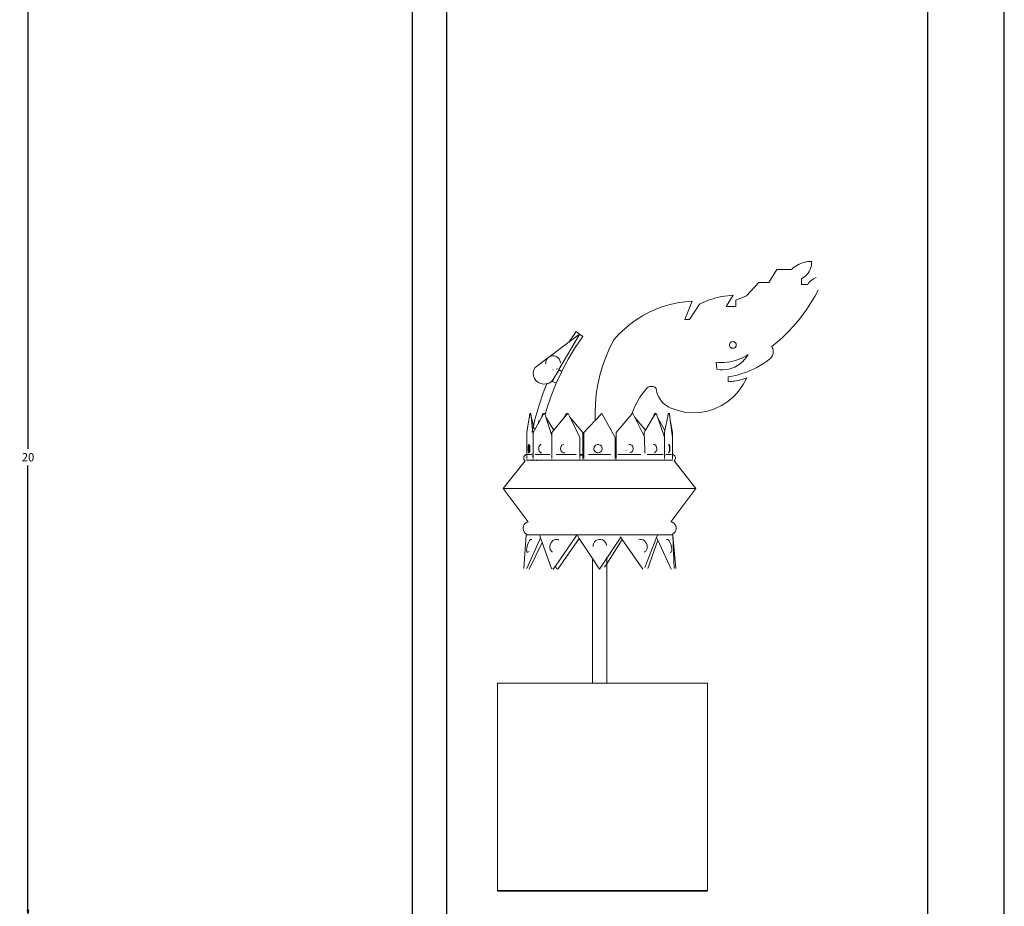
# Model space of a CAD drawing. Units: millimetres. Extents: x 446512 to 447461, y 70395 to 70610.
# Tile 4 of 39: x 446678.04 to 446699.43, y 70453.63 to 70472.88. Entities that reach past the tile are written whole.
import ezdxf

# ---------------------------------------------------------------- set-up
doc = ezdxf.new("R2010")
doc.units = ezdxf.units.MM
for name, color, linetype, lineweight in [('A-ANNO-DIMS', 2, 'Continuous', 18), ('A-FURN', 7, 'Continuous', 35), ('A-FURN-DECO', 8, 'Continuous', 13)]:
    doc.layers.add(name, color=color, linetype=linetype, lineweight=lineweight)
doc.styles.get("Standard").update_dxf_attribs({"font": 'arial.ttf'})
doc.dimstyles.get("Standard").update_dxf_attribs({"dimtxt": 0.18, "dimasz": 0.18, "dimexe": 0.18, "dimexo": 0.0625, "dimgap": 0.09, "dimtad": 0, "dimtih": 1, "dimtoh": 1, "dimdec": 4, "dimzin": 0, "dimdsep": 46, "dimtxsty": 'Standard', "dimcen": 0.09, "dimadec": 0, "dimazin": 0, "dimtfac": 1, "dimtdec": 4, "dimtofl": 0, "dimtmove": 0, "dimatfit": 3, "dimfxl": 1, "dimtolj": 1, "dimtzin": 0, "dimarcsym": 0})

# ---------------------------------------------------------------- blocks, each defined once
blk = doc.blocks.new('*D20')
at = {"layer": 'A-ANNO-DIMS', "color": 0, "lineweight": -2, "transparency": 16777216}
for p, q in [((446686.51, 70473.382), (446678.043, 70473.382)), ((446678.223, 70473.202), (446678.223, 70463.563)), ((446678.223, 70453.562), (446678.223, 70463.2)), ((446686.51, 70453.382), (446678.043, 70453.382))]:
    blk.add_line(p, q, dxfattribs=at)
at = {"layer": 'A-ANNO-DIMS', "color": 0, "transparency": 16777216}
for points in [[(446678.193, 70473.202), (446678.253, 70473.202), (446678.223, 70473.382)], [(446678.193, 70453.562), (446678.253, 70453.562), (446678.223, 70453.382)]]:
    blk.add_solid(points, dxfattribs=at)
at = {"layer": 'Defpoints', "color": 0, "transparency": 16777216}
for p in [(446678.223, 70473.382), (446686.573, 70473.382), (446686.573, 70453.382)]:
    blk.add_point(p, dxfattribs=at)
at = {"layer": 'A-ANNO-DIMS', "color": 0, "transparency": 16777216, "insert": (446678.223, 70463.382), "char_height": 0.18, "attachment_point": 5}
blk.add_mtext('\\A1;20', dxfattribs=at)
blk = doc.blocks.new('*D37')
at = {"layer": 'A-ANNO-DIMS', "color": 0, "lineweight": -2, "transparency": 16777216}
for p, q in [((446686.572846, 70433.44405), (446686.572846, 70578.17492)), ((446687.323552, 70428.838404), (446687.323552, 70578.17492)), ((446686.392846, 70577.99492), (446686.212846, 70577.99492)), ((446687.503552, 70577.99492), (446687.683552, 70577.99492))]:
    blk.add_line(p, q, dxfattribs=at)
at = {"layer": 'A-ANNO-DIMS', "color": 0, "transparency": 16777216}
for points in [[(446686.392846, 70578.02492), (446686.392846, 70577.96492), (446686.572846, 70577.99492)], [(446687.503552, 70578.02492), (446687.503552, 70577.96492), (446687.323552, 70577.99492)]]:
    blk.add_solid(points, dxfattribs=at)
at = {"layer": 'Defpoints', "color": 0, "transparency": 16777216}
for p in [(446687.323552, 70577.99492), (446686.572846, 70433.38155), (446687.323552, 70428.775904)]:
    blk.add_point(p, dxfattribs=at)
at = {"layer": 'A-ANNO-DIMS', "color": 0, "transparency": 16777216, "insert": (446686.948199, 70577.99492), "char_height": 0.18, "attachment_point": 5}
blk.add_mtext('\\A1;0.75', dxfattribs=at)
blk = doc.blocks.new('*D38')
at = {"layer": 'A-ANNO-DIMS', "color": 0, "lineweight": -2, "transparency": 16777216}
for p, q in [((446687.323552, 70428.838404), (446687.323552, 70578.17492)), ((446697.765686, 70428.838404), (446697.765686, 70578.17492)), ((446687.503552, 70577.99492), (446692.090383, 70577.99492)), ((446697.585686, 70577.99492), (446692.998855, 70577.99492))]:
    blk.add_line(p, q, dxfattribs=at)
at = {"layer": 'A-ANNO-DIMS', "color": 0, "transparency": 16777216}
for points in [[(446687.503552, 70578.02492), (446687.503552, 70577.96492), (446687.323552, 70577.99492)], [(446697.585686, 70578.02492), (446697.585686, 70577.96492), (446697.765686, 70577.99492)]]:
    blk.add_solid(points, dxfattribs=at)
at = {"layer": 'Defpoints', "color": 0, "transparency": 16777216}
for p in [(446697.765686, 70577.99492), (446687.323552, 70428.775904), (446697.765686, 70428.775904)]:
    blk.add_point(p, dxfattribs=at)
at = {"layer": 'A-ANNO-DIMS', "color": 0, "transparency": 16777216, "insert": (446692.544619, 70577.99492), "char_height": 0.18, "attachment_point": 5}
blk.add_mtext('\\A1;10.442', dxfattribs=at)
blk = doc.blocks.new('*D39')
at = {"layer": 'A-ANNO-DIMS', "color": 0, "lineweight": -2, "transparency": 16777216}
for p, q in [((446697.766, 70428.838), (446697.766, 70578.175)), ((446699.429, 70433.444), (446699.429, 70578.175)), ((446697.946, 70577.995), (446698.212, 70577.995)), ((446699.249, 70577.995), (446698.982, 70577.995))]:
    blk.add_line(p, q, dxfattribs=at)
at = {"layer": 'A-ANNO-DIMS', "color": 0, "transparency": 16777216}
for points in [[(446697.946, 70578.025), (446697.946, 70577.965), (446697.766, 70577.995)], [(446699.249, 70578.025), (446699.249, 70577.965), (446699.429, 70577.995)]]:
    blk.add_solid(points, dxfattribs=at)
at = {"layer": 'Defpoints', "color": 0, "transparency": 16777216}
for p in [(446699.429, 70577.995), (446699.429, 70433.382), (446697.766, 70428.776)]:
    blk.add_point(p, dxfattribs=at)
at = {"layer": 'A-ANNO-DIMS', "color": 0, "transparency": 16777216, "insert": (446698.597, 70577.995), "char_height": 0.18, "attachment_point": 5}
blk.add_mtext('\\A1;1.663', dxfattribs=at)

msp = doc.modelspace()

# ---------------------------------------------------------------- linework, layer by layer
at = {"layer": 'A-FURN'}
msp.add_line((446688.42, 70453.9655), (446692.9826, 70453.9655), dxfattribs=at)
at = {"layer": 'A-FURN-DECO'}
for p, q in [((446694.3144, 70467.1785), (446694.4873, 70467.4578)), ((446694.4873, 70467.4578), (446694.8067, 70467.4578)), ((446694.8067, 70467.4578), (446694.8365, 70467.4847)), ((446694.8365, 70467.4847), (446694.8679, 70467.5096)), ((446694.8679, 70467.5096), (446694.9009, 70467.5324)), ((446694.9009, 70467.5324), (446694.9353, 70467.5531)), ((446694.9353, 70467.5531), (446694.9709, 70467.5716)), ((446694.9709, 70467.5716), (446695.0077, 70467.5878)), ((446695.0077, 70467.5878), (446695.0454, 70467.6015)), ((446695.0454, 70467.6015), (446695.0839, 70467.6129)), ((446695.0839, 70467.6129), (446695.123, 70467.6217)), ((446695.123, 70467.6217), (446695.1627, 70467.6281)), ((446695.1627, 70467.6281), (446695.2026, 70467.6319)), ((446695.2053, 70467.4459), (446695.1875, 70467.4117)), ((446695.2026, 70467.6319), (446695.2427, 70467.6331)), ((446695.2199, 70467.4816), (446695.2053, 70467.4459)), ((446695.2309, 70467.5185), (446695.2199, 70467.4816)), ((446695.2385, 70467.5562), (446695.2309, 70467.5185)), ((446695.2424, 70467.5946), (446695.2385, 70467.5562)), ((446695.2427, 70467.6331), (446695.2424, 70467.5946)), ((446695.0554, 70467.274), (446695.022, 70467.2548)), ((446695.022, 70467.2548), (446695.022, 70467.1316)), ((446695.0868, 70467.2963), (446695.0554, 70467.274)), ((446695.116, 70467.3214), (446695.0868, 70467.2963)), ((446695.1426, 70467.3492), (446695.116, 70467.3214)), ((446695.1666, 70467.3794), (446695.1426, 70467.3492)), ((446695.1875, 70467.4117), (446695.1666, 70467.3794)), ((446695.2254, 70467.2123), (446695.2525, 70467.2346)), ((446695.2525, 70467.2346), (446695.2816, 70467.2541)), ((446695.2816, 70467.2541), (446695.3124, 70467.2707)), ((446695.3124, 70467.2707), (446695.3446, 70467.2842)), ((446693.8287, 70466.8825), (446694.0999, 70467.1785)), ((446694.0999, 70467.1785), (446694.3144, 70467.1785)), ((446695.022, 70467.1316), (446695.1589, 70467.1316)), ((446695.1589, 70467.1316), (446695.1784, 70467.1606)), ((446695.1784, 70467.1606), (446695.2007, 70467.1876)), ((446695.2007, 70467.1876), (446695.2254, 70467.2123)), ((446692.9818, 70466.7815), (446693.042, 70466.8034)), ((446693.042, 70466.8034), (446693.1028, 70466.8231)), ((446693.1028, 70466.8231), (446693.1644, 70466.8406)), ((446693.1644, 70466.8406), (446693.2265, 70466.8559)), ((446693.2265, 70466.8559), (446693.2891, 70466.869)), ((446693.2891, 70466.869), (446693.3522, 70466.8798)), ((446693.3522, 70466.8798), (446693.4156, 70466.8884)), ((446693.5431, 70466.8987), (446693.3856, 70466.6528)), ((446693.4156, 70466.8884), (446693.4793, 70466.8947)), ((446693.4793, 70466.8947), (446693.5431, 70466.8987)), ((446693.5955, 70466.7897), (446693.8287, 70466.8825)), ((446695.3111, 70466.8693), (446695.2297, 70466.7314)), ((446695.3861, 70467.0106), (446695.3111, 70466.8693)), ((446691.7134, 70466.5282), (446691.8616, 70466.5952)), ((446691.8616, 70466.5952), (446692.014, 70466.6519)), ((446692.014, 70466.6519), (446692.1699, 70466.6981)), ((446692.1699, 70466.6981), (446692.3286, 70466.7337)), ((446692.3286, 70466.7337), (446692.4893, 70466.7584)), ((446692.4893, 70466.7584), (446692.6513, 70466.7721)), ((446692.6513, 70466.7721), (446692.4922, 70466.3689)), ((446692.5926, 70466.3689), (446692.8067, 70466.7032)), ((446692.8067, 70466.7032), (446692.8641, 70466.7314)), ((446692.8641, 70466.7314), (446692.9225, 70466.7575)), ((446692.9225, 70466.7575), (446692.9818, 70466.7815)), ((446693.3856, 70466.6528), (446693.5955, 70466.6528)), ((446693.5955, 70466.6528), (446693.5955, 70466.7897)), ((446695.1424, 70466.5973), (446695.0491, 70466.4672)), ((446695.2297, 70466.7314), (446695.1424, 70466.5973)), ((446691.4323, 70466.365), (446691.5701, 70466.4514)), ((446691.5701, 70466.4514), (446691.7134, 70466.5282)), ((446695.0491, 70466.4672), (446694.9501, 70466.3414)), ((446691.0586, 70466.0527), (446691.176, 70466.1652)), ((446691.176, 70466.1652), (446691.3008, 70466.2695)), ((446691.3008, 70466.2695), (446691.4323, 70466.365)), ((446692.4922, 70466.3689), (446692.5926, 70466.3689)), ((446694.8456, 70466.2202), (446694.7359, 70466.1037)), ((446694.9501, 70466.3414), (446694.8456, 70466.2202)), ((446690.202, 70466.0449), (446689.7562, 70465.2847)), ((446690.1268, 70466.1082), (446689.9751, 70465.8868)), ((446690.202, 70466.0567), (446689.9751, 70465.8868)), ((446690.1103, 70465.7614), (446690.2773, 70466.0051)), ((446690.202, 70466.0567), (446690.1268, 70466.1082)), ((446690.202, 70466.0449), (446690.202, 70466.0567)), ((446690.2773, 70466.0051), (446690.202, 70466.0567)), ((446690.9491, 70465.9325), (446691.0586, 70466.0527)), ((446694.621, 70465.9922), (446694.5013, 70465.886)), ((446694.7359, 70466.1037), (446694.621, 70465.9922)), ((446689.9751, 70465.8868), (446689.5362, 70465.5564)), ((446689.9581, 70465.511), (446690.1103, 70465.7614)), ((446690.8555, 70465.7475), (446690.7735, 70465.557)), ((446690.9491, 70465.9325), (446690.8555, 70465.7475)), ((446693.4621, 70465.8096), (446693.4622, 70465.8286)), ((446693.467, 70465.7911), (446693.4621, 70465.8096)), ((446693.4622, 70465.8286), (446693.4673, 70465.847)), ((446693.4764, 70465.7746), (446693.467, 70465.7911)), ((446693.4673, 70465.847), (446693.4769, 70465.8635)), ((446693.4898, 70465.761), (446693.4764, 70465.7746)), ((446693.4769, 70465.8635), (446693.4904, 70465.8769)), ((446693.5063, 70465.7514), (446693.4898, 70465.761)), ((446693.4904, 70465.8769), (446693.507, 70465.8863)), ((446693.5247, 70465.7464), (446693.5063, 70465.7514)), ((446693.507, 70465.8863), (446693.5254, 70465.8911)), ((446693.5437, 70465.7463), (446693.5247, 70465.7464)), ((446693.5254, 70465.8911), (446693.5445, 70465.891)), ((446693.5622, 70465.7511), (446693.5437, 70465.7463)), ((446693.5445, 70465.891), (446693.5628, 70465.886)), ((446693.5787, 70465.7606), (446693.5622, 70465.7511)), ((446693.5628, 70465.886), (446693.5793, 70465.8764)), ((446693.5922, 70465.774), (446693.5787, 70465.7606)), ((446693.5793, 70465.8764), (446693.5927, 70465.8629)), ((446693.6019, 70465.7904), (446693.5922, 70465.774)), ((446693.5927, 70465.8629), (446693.6022, 70465.8463)), ((446693.6069, 70465.8088), (446693.6019, 70465.7904)), ((446693.6022, 70465.8463), (446693.607, 70465.8279)), ((446693.607, 70465.8279), (446693.6069, 70465.8088)), ((446694.5013, 70465.886), (446694.3769, 70465.7852)), ((446694.3769, 70465.7852), (446694.3896, 70465.7631)), ((446694.3896, 70465.7631), (446694.3995, 70465.7396)), ((446694.3995, 70465.7396), (446694.4063, 70465.715)), ((446689.5362, 70465.5564), (446689.2354, 70465.3333)), ((446689.4825, 70465.4957), (446689.5052, 70465.5294)), ((446689.5052, 70465.5294), (446689.5362, 70465.5564)), ((446689.5362, 70465.5564), (446689.5733, 70465.5747)), ((446689.5733, 70465.5747), (446689.6141, 70465.583)), ((446689.6141, 70465.583), (446689.6557, 70465.5809)), ((446689.6557, 70465.5809), (446689.6954, 70465.5684)), ((446689.6954, 70465.5684), (446689.7303, 70465.5465)), ((446689.7303, 70465.5465), (446689.7582, 70465.5166)), ((446690.7735, 70465.557), (446690.7035, 70465.3618)), ((446693.7029, 70465.524), (446693.6465, 70465.5011)), ((446693.758, 70465.5502), (446693.7029, 70465.524)), ((446693.8114, 70465.5795), (446693.758, 70465.5502)), ((446693.8278, 70465.5548), (446693.7869, 70465.5017)), ((446693.8629, 70465.612), (446693.8114, 70465.5795)), ((446693.8629, 70465.612), (446693.8278, 70465.5548)), ((446694.3503, 70465.5275), (446694.3311, 70465.5107)), ((446694.3673, 70465.5465), (446694.3503, 70465.5275)), ((446694.3817, 70465.5675), (446694.3673, 70465.5465)), ((446694.3934, 70465.5902), (446694.3817, 70465.5675)), ((446694.4023, 70465.6141), (446694.3934, 70465.5902)), ((446694.408, 70465.6389), (446694.4023, 70465.6141)), ((446694.4063, 70465.715), (446694.4101, 70465.6898)), ((446694.4106, 70465.6643), (446694.408, 70465.6389)), ((446694.4101, 70465.6898), (446694.4106, 70465.6643)), ((446689.2354, 70465.3333), (446689.2086, 70465.2796)), ((446689.4674, 70465.4172), (446689.4696, 70465.4574)), ((446689.4677, 70465.4158), (446689.4674, 70465.4172)), ((446689.4674, 70465.4101), (446689.4677, 70465.4158)), ((446689.4696, 70465.4574), (446689.4825, 70465.4957)), ((446689.7582, 70465.5166), (446689.7771, 70465.4807)), ((446689.7771, 70465.4807), (446689.7858, 70465.4413)), ((446689.7855, 70465.4356), (446689.7858, 70465.4413)), ((446689.7855, 70465.4356), (446689.7858, 70465.4342)), ((446689.9581, 70465.511), (446689.8195, 70465.2529)), ((446690.7035, 70465.3618), (446690.6456, 70465.1627)), ((446693.2276, 70465.4378), (446693.1668, 70465.443)), ((446693.1668, 70465.443), (446693.1818, 70465.2914)), ((446693.2885, 70465.4362), (446693.2276, 70465.4378)), ((446693.3494, 70465.4382), (446693.2885, 70465.4362)), ((446693.4101, 70465.4437), (446693.3494, 70465.4382)), ((446693.4703, 70465.4528), (446693.4101, 70465.4437)), ((446693.5127, 70465.3149), (446693.4483, 70465.2963)), ((446693.53, 70465.4654), (446693.4703, 70465.4528)), ((446693.5748, 70465.3403), (446693.5127, 70465.3149)), ((446693.5887, 70465.4816), (446693.53, 70465.4654)), ((446693.6339, 70465.372), (446693.5748, 70465.3403)), ((446693.6465, 70465.5011), (446693.5887, 70465.4816)), ((446693.6894, 70465.4098), (446693.6339, 70465.372)), ((446693.7406, 70465.4532), (446693.6894, 70465.4098)), ((446693.7869, 70465.5017), (446693.7406, 70465.4532)), ((446694.0548, 70465.3329), (446693.9814, 70465.2959)), ((446694.1266, 70465.373), (446694.0548, 70465.3329)), ((446694.1967, 70465.416), (446694.1266, 70465.373)), ((446694.2649, 70465.4619), (446694.1967, 70465.416)), ((446694.3311, 70465.5107), (446694.2649, 70465.4619)), ((446689.2086, 70465.2796), (446689.197, 70465.221)), ((446689.197, 70465.2092), (446689.197, 70465.221)), ((446689.197, 70465.2092), (446689.2016, 70465.1498)), ((446689.2016, 70465.1498), (446689.2219, 70465.0935)), ((446689.2219, 70465.0935), (446689.2566, 70465.0442)), ((446689.6439, 70465.0931), (446689.6134, 70465.0281)), ((446689.6288, 70465.276), (446689.6256, 70465.2691)), ((446689.7498, 70465.2738), (446689.6308, 70465.0709)), ((446689.696, 70464.9894), (446689.815, 70465.2433)), ((446689.7036, 70465.2955), (446689.711, 70465.292)), ((446689.7238, 70465.3009), (446689.7187, 70465.3035)), ((446689.7562, 70465.2847), (446689.7498, 70465.2738)), ((446689.815, 70465.2433), (446689.7498, 70465.2738)), ((446689.7562, 70465.2847), (446689.8195, 70465.2529)), ((446690.6456, 70465.1627), (446690.6002, 70464.9604)), ((446693.2482, 70465.2821), (446693.1818, 70465.2914)), ((446693.3153, 70465.2797), (446693.2482, 70465.2821)), ((446693.3822, 70465.2845), (446693.3153, 70465.2797)), ((446693.4483, 70465.2963), (446693.3822, 70465.2845)), ((446693.5143, 70465.1411), (446693.4333, 70465.1269)), ((446693.4333, 70465.1269), (446693.4333, 70465.022)), ((446693.5946, 70465.1586), (446693.5143, 70465.1411)), ((446693.6741, 70465.1795), (446693.5946, 70465.1586)), ((446693.7527, 70465.2038), (446693.6741, 70465.1795)), ((446693.8302, 70465.2313), (446693.7527, 70465.2038)), ((446693.835, 70465.1072), (446693.7595, 70464.9596)), ((446693.7705, 70465.0831), (446693.8029, 70465.0947)), ((446693.8029, 70465.0947), (446693.835, 70465.1072)), ((446693.9065, 70465.262), (446693.8302, 70465.2313)), ((446693.9814, 70465.2959), (446693.9065, 70465.262)), ((446689.2566, 70465.0442), (446689.3034, 70465.0052)), ((446689.3034, 70465.0052), (446689.359, 70464.9793)), ((446689.359, 70464.9793), (446689.4196, 70464.9682)), ((446689.494, 70464.9769), (446689.4143, 70464.7798)), ((446689.4196, 70464.9682), (446689.4812, 70464.9725)), ((446689.4812, 70464.9725), (446689.494, 70464.9769)), ((446689.494, 70464.9769), (446689.5395, 70464.9922)), ((446689.4995, 70464.9905), (446689.494, 70464.9769)), ((446689.5395, 70464.9922), (446689.5905, 70465.0257)), ((446689.5853, 70464.7159), (446689.6952, 70464.9876)), ((446689.5866, 70465.0349), (446689.5953, 70465.0311)), ((446689.5905, 70465.0257), (446689.5953, 70465.0311)), ((446689.5988, 70465.035), (446689.592, 70465.0381)), ((446689.5953, 70465.0311), (446689.5988, 70465.035)), ((446689.5953, 70465.0311), (446689.6952, 70464.9876)), ((446689.5988, 70465.035), (446689.6308, 70465.0709)), ((446689.5988, 70465.035), (446689.696, 70464.9894)), ((446689.6134, 70465.0281), (446689.6115, 70465.0241)), ((446690.6002, 70464.9604), (446690.5673, 70464.7557)), ((446691.6745, 70464.8887), (446691.6606, 70464.8754)), ((446691.6901, 70464.9), (446691.6745, 70464.8887)), ((446691.7071, 70464.9091), (446691.6901, 70464.9)), ((446691.7252, 70464.9156), (446691.7071, 70464.9091)), ((446691.744, 70464.9196), (446691.7252, 70464.9156)), ((446691.7632, 70464.921), (446691.744, 70464.9196)), ((446691.7825, 70464.9196), (446691.7632, 70464.921)), ((446691.8013, 70464.9156), (446691.7825, 70464.9196)), ((446691.8194, 70464.9091), (446691.8013, 70464.9156)), ((446691.8364, 70464.9), (446691.8194, 70464.9091)), ((446691.852, 70464.8887), (446691.8364, 70464.9)), ((446691.8659, 70464.8754), (446691.852, 70464.8887)), ((446693.4333, 70465.022), (446693.4676, 70465.0236)), ((446693.4676, 70465.0236), (446693.5019, 70465.0262)), ((446693.5019, 70465.0262), (446693.5362, 70465.0298)), ((446693.5362, 70465.0298), (446693.5702, 70465.0344)), ((446693.5702, 70465.0344), (446693.6042, 70465.0401)), ((446693.6042, 70465.0401), (446693.6379, 70465.0467)), ((446693.6379, 70465.0467), (446693.6715, 70465.0543)), ((446693.7595, 70464.9596), (446693.6652, 70464.8233)), ((446693.6715, 70465.0543), (446693.7048, 70465.063)), ((446693.7048, 70465.063), (446693.7378, 70465.0726)), ((446693.7378, 70465.0726), (446693.7705, 70465.0831)), ((446689.4143, 70464.7798), (446689.316, 70464.4933)), ((446689.4903, 70464.4388), (446689.5853, 70464.7159)), ((446690.5673, 70464.7557), (446690.5472, 70464.5493)), ((446691.5135, 70464.684), (446691.4517, 70464.5802)), ((446691.5832, 70464.7826), (446691.5135, 70464.684)), ((446691.6606, 70464.8754), (446691.5832, 70464.7826)), ((446691.8725, 70464.8309), (446691.8659, 70464.8754)), ((446691.883, 70464.7871), (446691.8725, 70464.8309)), ((446691.8972, 70464.7445), (446691.883, 70464.7871)), ((446691.9151, 70464.7032), (446691.8972, 70464.7445)), ((446691.9366, 70464.6637), (446691.9151, 70464.7032)), ((446691.9613, 70464.6262), (446691.9366, 70464.6637)), ((446693.5538, 70464.7005), (446693.4273, 70464.5935)), ((446693.6652, 70464.8233), (446693.5538, 70464.7005)), ((446689.316, 70464.4933), (446689.2335, 70464.2019)), ((446690.5472, 70464.5493), (446690.5398, 70464.3421)), ((446691.3983, 70464.4718), (446691.3536, 70464.3596)), ((446691.4517, 70464.5802), (446691.3983, 70464.4718)), ((446691.9893, 70464.5909), (446691.9613, 70464.6262)), ((446692.0202, 70464.5583), (446691.9893, 70464.5909)), ((446692.0538, 70464.5284), (446692.0202, 70464.5583)), ((446692.0899, 70464.5016), (446692.0538, 70464.5284)), ((446692.1282, 70464.478), (446692.0899, 70464.5016)), ((446692.1685, 70464.4579), (446692.1282, 70464.478)), ((446692.3239, 70464.4003), (446692.1685, 70464.4579)), ((446693.2877, 70464.5041), (446693.1375, 70464.4339)), ((446693.4273, 70464.5935), (446693.2877, 70464.5041)), ((446689.1073, 70464.2199), (446689.1217, 70464.3336)), ((446689.1291, 70464.3336), (446689.1073, 70464.2199)), ((446689.1291, 70464.3336), (446689.1217, 70464.3336)), ((446689.1291, 70464.3336), (446689.147, 70464.3336)), ((446689.1538, 70464.2683), (446689.147, 70464.3336)), ((446689.1538, 70464.2683), (446689.2004, 70464.0558)), ((446689.1836, 70463.9812), (446689.1538, 70464.2683)), ((446689.3746, 70464.2352), (446689.1955, 70463.9194)), ((446689.3746, 70464.2352), (446689.4088, 70464.3336)), ((446689.4304, 70464.3336), (446689.3746, 70464.2352)), ((446689.413, 70464.3336), (446689.4088, 70464.3336)), ((446689.445, 70464.3336), (446689.4304, 70464.3336)), ((446689.4533, 70464.3084), (446689.445, 70464.3336)), ((446689.4533, 70464.3084), (446689.4903, 70464.4388)), ((446689.4718, 70464.2521), (446689.4533, 70464.3084)), ((446689.4718, 70464.2521), (446689.6426, 70463.9673)), ((446689.6027, 70463.8537), (446689.4718, 70464.2521)), ((446689.871, 70464.2417), (446689.6426, 70463.9673)), ((446689.871, 70464.2417), (446689.9164, 70464.3336)), ((446689.9361, 70464.3198), (446689.871, 70464.2417)), ((446689.9244, 70464.3336), (446689.9164, 70464.3336)), ((446689.9244, 70464.3336), (446689.9361, 70464.3198)), ((446689.9476, 70464.3336), (446689.9361, 70464.3198)), ((446689.9563, 70464.3336), (446689.9476, 70464.3336)), ((446689.998, 70464.2471), (446689.9563, 70464.3336)), ((446689.978, 70464.2707), (446689.998, 70464.2471)), ((446689.998, 70464.2471), (446690.2771, 70463.9194)), ((446690.2072, 70463.8135), (446689.998, 70464.2471)), ((446690.5398, 70464.3421), (446690.5441, 70464.1801)), ((446690.6894, 70464.3336), (446690.5441, 70464.1801)), ((446690.9746, 70463.8135), (446690.6894, 70464.3336)), ((446691.3409, 70464.3187), (446690.9991, 70463.9194)), ((446691.3409, 70464.3187), (446691.3375, 70464.3074)), ((446691.342, 70464.3221), (446691.3409, 70464.3187)), ((446691.3409, 70464.3187), (446691.344, 70464.3151)), ((446691.3536, 70464.3596), (446691.342, 70464.3221)), ((446691.3518, 70464.3336), (446691.342, 70464.3221)), ((446691.3518, 70464.3336), (446691.3597, 70464.3336)), ((446691.4051, 70464.2417), (446691.3597, 70464.3336)), ((446691.4051, 70464.2417), (446691.6336, 70463.9673)), ((446691.4051, 70464.2417), (446691.6049, 70463.8368)), ((446691.8043, 70464.2521), (446691.6336, 70463.9673)), ((446691.8043, 70464.2521), (446691.8311, 70464.3336)), ((446691.8494, 70464.3272), (446691.8043, 70464.2521)), ((446691.8311, 70464.3336), (446691.8457, 70464.3336)), ((446691.8457, 70464.3336), (446691.8494, 70464.3272)), ((446691.8532, 70464.3336), (446691.8494, 70464.3272)), ((446691.8532, 70464.3336), (446691.8673, 70464.3336)), ((446691.9015, 70464.2352), (446691.8673, 70464.3336)), ((446691.9015, 70464.2352), (446692.0555, 70463.9637)), ((446691.9015, 70464.2352), (446692.0458, 70463.8199)), ((446692.1223, 70464.2683), (446692.0555, 70463.9637)), ((446692.1223, 70464.2683), (446692.1291, 70464.3336)), ((446692.1367, 70464.3336), (446692.1223, 70464.2683)), ((446692.1291, 70464.3336), (446692.1367, 70464.3336)), ((446692.1367, 70464.3336), (446692.1544, 70464.3336)), ((446692.1544, 70464.3336), (446692.1725, 70464.1914)), ((446692.4855, 70464.3636), (446692.3239, 70464.4003)), ((446692.6506, 70464.3486), (446692.4855, 70464.3636)), ((446692.8162, 70464.3555), (446692.6506, 70464.3486)), ((446692.9795, 70464.3841), (446692.8162, 70464.3555)), ((446693.1375, 70464.4339), (446692.9795, 70464.3841)), ((446689.1037, 70464.1914), (446689.055, 70463.9194)), ((446689.1037, 70464.1914), (446689.1073, 70464.2199)), ((446689.2004, 70464.0558), (446689.1836, 70463.9812)), ((446689.2335, 70464.2019), (446689.2004, 70464.0558)), ((446689.2004, 70464.0558), (446689.2139, 70463.9942)), ((446689.3219, 70464.1794), (446689.308, 70464.1177)), ((446690.5441, 70464.1801), (446690.2973, 70463.9194)), ((446692.1725, 70464.1914), (446692.2212, 70463.9194)), ((446692.2205, 70463.8135), (446692.1725, 70464.1914)), ((446689.0556, 70463.8135), (446689.0549, 70463.442)), ((446689.055, 70463.9194), (446689.0565, 70463.82)), ((446689.0556, 70463.8135), (446689.0565, 70463.82)), ((446689.1836, 70463.9812), (446689.1713, 70463.9268)), ((446689.1955, 70463.866), (446689.1836, 70463.9812)), ((446689.1955, 70463.9194), (446689.1955, 70463.866)), ((446689.1955, 70463.866), (446689.1955, 70463.4432)), ((446689.6426, 70463.9673), (446689.6027, 70463.9194)), ((446689.6027, 70463.9194), (446689.6027, 70463.8537)), ((446689.6027, 70463.8537), (446689.6027, 70463.4381)), ((446690.2072, 70463.8135), (446690.21, 70463.4432)), ((446690.2771, 70463.9194), (446690.2771, 70463.4432)), ((446690.2973, 70463.9194), (446690.2973, 70463.4432)), ((446690.9746, 70463.8135), (446690.9771, 70463.5235)), ((446690.9991, 70463.9194), (446690.9991, 70463.5237)), ((446691.6336, 70463.9673), (446691.6049, 70463.9194)), ((446691.6049, 70463.9194), (446691.6049, 70463.8368)), ((446691.6163, 70463.8135), (446691.6049, 70463.8368)), ((446691.6163, 70463.8135), (446691.619, 70463.4712)), ((446692.0555, 70463.9637), (446692.0458, 70463.9194)), ((446692.0458, 70463.9194), (446692.0458, 70463.8199)), ((446692.048, 70463.8135), (446692.0458, 70463.8199)), ((446692.048, 70463.8135), (446692.05, 70463.4432)), ((446692.2212, 70463.9194), (446692.2205, 70463.8135)), ((446692.2205, 70463.8135), (446692.2213, 70463.442)), ((446689.087, 70463.5804), (446689.0882, 70463.6033)), ((446689.0882, 70463.6033), (446689.0905, 70463.6239)), ((446689.0905, 70463.6239), (446689.0937, 70463.6407)), ((446689.0937, 70463.6407), (446689.0976, 70463.6526)), ((446689.096, 70463.5804), (446689.0972, 70463.6033)), ((446689.0972, 70463.6033), (446689.0995, 70463.6239)), ((446689.0976, 70463.6526), (446689.1019, 70463.6587)), ((446689.0995, 70463.6239), (446689.1026, 70463.6407)), ((446689.1109, 70463.6587), (446689.1019, 70463.6587)), ((446689.1026, 70463.6407), (446689.1066, 70463.6526)), ((446689.1066, 70463.6526), (446689.1109, 70463.6587)), ((446689.1129, 70463.6029), (446689.1115, 70463.5799)), ((446689.1157, 70463.6236), (446689.1129, 70463.6029)), ((446689.1161, 70463.6079), (446689.1129, 70463.6029)), ((446689.1196, 70463.6404), (446689.1157, 70463.6236)), ((446689.1157, 70463.6236), (446689.1161, 70463.6079)), ((446689.1218, 70463.6461), (446689.1196, 70463.6404)), ((446689.1223, 70463.6446), (446689.1196, 70463.6404)), ((446689.1218, 70463.6029), (446689.1204, 70463.5799)), ((446689.1245, 70463.6236), (446689.1218, 70463.6029)), ((446689.1258, 70463.629), (446689.1245, 70463.6236)), ((446689.3182, 70463.5804), (446689.322, 70463.6033)), ((446689.322, 70463.6033), (446689.3291, 70463.6239)), ((446689.3291, 70463.6239), (446689.3392, 70463.6407)), ((446689.3392, 70463.6407), (446689.3516, 70463.6526)), ((446689.3516, 70463.6526), (446689.3654, 70463.6587)), ((446689.3727, 70463.6587), (446689.3654, 70463.6587)), ((446689.7893, 70463.5804), (446689.7947, 70463.6033)), ((446689.7947, 70463.6033), (446689.8053, 70463.6239)), ((446689.8053, 70463.6239), (446689.8201, 70463.6407)), ((446689.8201, 70463.6407), (446689.8383, 70463.6526)), ((446689.8383, 70463.6526), (446689.8585, 70463.6587)), ((446689.8629, 70463.6587), (446689.8585, 70463.6587)), ((446690.5143, 70463.5804), (446690.5205, 70463.6033)), ((446690.5205, 70463.6033), (446690.5325, 70463.6239)), ((446690.5325, 70463.6239), (446690.5494, 70463.6407)), ((446690.5494, 70463.6407), (446690.57, 70463.6526)), ((446690.57, 70463.6526), (446690.593, 70463.6587)), ((446690.593, 70463.6587), (446690.6169, 70463.6586)), ((446690.6169, 70463.6586), (446690.6399, 70463.6524)), ((446690.6399, 70463.6524), (446690.6605, 70463.6404)), ((446690.6605, 70463.6404), (446690.6773, 70463.6236)), ((446690.6773, 70463.6236), (446690.6891, 70463.6029)), ((446690.6891, 70463.6029), (446690.6952, 70463.5799)), ((446691.2731, 70463.6587), (446691.2771, 70463.6587)), ((446691.2771, 70463.6587), (446691.2985, 70463.6586)), ((446691.2985, 70463.6586), (446691.3192, 70463.6524)), ((446691.3192, 70463.6524), (446691.3377, 70463.6404)), ((446691.3377, 70463.6404), (446691.3528, 70463.6236)), ((446691.3528, 70463.6236), (446691.3635, 70463.6029)), ((446691.3635, 70463.6029), (446691.369, 70463.5799)), ((446691.8063, 70463.6587), (446691.8134, 70463.6587)), ((446691.8134, 70463.6587), (446691.8285, 70463.6586)), ((446691.8285, 70463.6586), (446691.8431, 70463.6524)), ((446691.8431, 70463.6524), (446691.8561, 70463.6404)), ((446691.8561, 70463.6404), (446691.8667, 70463.6236)), ((446691.8667, 70463.6236), (446691.8743, 70463.6029)), ((446691.8743, 70463.6029), (446691.8781, 70463.5799)), ((446692.1321, 70463.6587), (446692.1376, 70463.6586)), ((446692.1376, 70463.6586), (446692.141, 70463.6587)), ((446692.1376, 70463.6586), (446692.1429, 70463.6524)), ((446692.141, 70463.6587), (446692.1465, 70463.6586)), ((446692.1429, 70463.6524), (446692.1477, 70463.6404)), ((446692.1465, 70463.6586), (446692.1518, 70463.6524)), ((446692.1477, 70463.6404), (446692.1516, 70463.6236)), ((446692.1516, 70463.6236), (446692.1544, 70463.6029)), ((446692.1518, 70463.6524), (446692.1566, 70463.6404)), ((446692.1544, 70463.6029), (446692.1558, 70463.5799)), ((446692.1566, 70463.6404), (446692.1605, 70463.6236)), ((446692.1605, 70463.6236), (446692.1632, 70463.6029)), ((446692.1632, 70463.6029), (446692.1646, 70463.5799)), ((446688.9899, 70463.3755), (446688.9955, 70463.3955)), ((446688.9955, 70463.3955), (446689.0062, 70463.4134)), ((446689.0062, 70463.4134), (446689.0212, 70463.428)), ((446689.0212, 70463.428), (446689.0394, 70463.4381)), ((446689.0394, 70463.4381), (446689.0549, 70463.442)), ((446689.0549, 70463.428), (446689.0547, 70463.3546)), ((446689.0549, 70463.442), (446689.0596, 70463.4432)), ((446689.0549, 70463.442), (446689.0549, 70463.4381)), ((446689.0596, 70463.4432), (446689.0631, 70463.4432)), ((446689.0596, 70463.4432), (446689.061, 70463.4432)), ((446689.1665, 70463.4432), (446689.0631, 70463.4432)), ((446689.087, 70463.5565), (446689.087, 70463.5804)), ((446689.0882, 70463.5335), (446689.087, 70463.5565)), ((446689.0904, 70463.5128), (446689.0882, 70463.5335)), ((446689.0936, 70463.496), (446689.0904, 70463.5128)), ((446689.0975, 70463.484), (446689.0936, 70463.496)), ((446689.096, 70463.5565), (446689.096, 70463.5804)), ((446689.0972, 70463.5335), (446689.096, 70463.5565)), ((446689.0994, 70463.5128), (446689.0972, 70463.5335)), ((446689.1019, 70463.4778), (446689.0975, 70463.484)), ((446689.1026, 70463.496), (446689.0994, 70463.5128)), ((446689.1064, 70463.4777), (446689.1019, 70463.4778)), ((446689.1115, 70463.556), (446689.1026, 70463.496)), ((446689.1065, 70463.484), (446689.1026, 70463.496)), ((446689.1108, 70463.4778), (446689.1064, 70463.4777)), ((446689.1108, 70463.4778), (446689.1065, 70463.484)), ((446689.1153, 70463.4777), (446689.1108, 70463.4778)), ((446689.1115, 70463.5799), (446689.1115, 70463.556)), ((446689.1115, 70463.556), (446689.113, 70463.5331)), ((446689.113, 70463.5331), (446689.1157, 70463.5125)), ((446689.1157, 70463.5125), (446689.1196, 70463.4957)), ((446689.1196, 70463.4957), (446689.1218, 70463.4903)), ((446689.1204, 70463.5799), (446689.1204, 70463.556)), ((446689.1204, 70463.556), (446689.1218, 70463.5331)), ((446689.1218, 70463.5331), (446689.1246, 70463.5125)), ((446689.1246, 70463.5125), (446689.1258, 70463.5073)), ((446689.1955, 70463.4432), (446689.1837, 70463.4432)), ((446689.1873, 70463.428), (446689.1837, 70463.3967)), ((446689.1955, 70463.4266), (446689.1837, 70463.4266)), ((446689.1955, 70463.4998), (446689.1885, 70463.4381)), ((446689.1955, 70463.4432), (446689.1955, 70463.4381)), ((446689.1955, 70463.428), (446689.1955, 70463.4266)), ((446689.1955, 70463.4266), (446689.1955, 70463.3546)), ((446689.5682, 70463.4432), (446689.2388, 70463.4432)), ((446689.3182, 70463.5565), (446689.3182, 70463.5804)), ((446689.3219, 70463.5335), (446689.3182, 70463.5565)), ((446689.329, 70463.5128), (446689.3219, 70463.5335)), ((446689.339, 70463.496), (446689.329, 70463.5128)), ((446689.3514, 70463.484), (446689.339, 70463.496)), ((446689.3651, 70463.4778), (446689.3514, 70463.484)), ((446689.3794, 70463.4777), (446689.3651, 70463.4778)), ((446689.3867, 70463.4777), (446689.3794, 70463.4777)), ((446689.6027, 70463.428), (446689.6027, 70463.3546)), ((446689.6917, 70463.4432), (446690.1304, 70463.4432)), ((446689.7892, 70463.5565), (446689.7893, 70463.5804)), ((446689.7946, 70463.5335), (446689.7892, 70463.5565)), ((446689.805, 70463.5128), (446689.7946, 70463.5335)), ((446689.8198, 70463.496), (446689.805, 70463.5128)), ((446689.8379, 70463.484), (446689.8198, 70463.496)), ((446689.8581, 70463.4778), (446689.8379, 70463.484)), ((446689.8791, 70463.4777), (446689.8581, 70463.4778)), ((446689.8834, 70463.4777), (446689.8791, 70463.4777)), ((446690.21, 70463.4432), (446690.2013, 70463.4432)), ((446690.2101, 70463.4266), (446690.2015, 70463.4266)), ((446690.21, 70463.4432), (446690.21, 70463.4381)), ((446690.2771, 70463.4432), (446690.21, 70463.4432)), ((446690.2101, 70463.428), (446690.2101, 70463.4266)), ((446690.2101, 70463.4266), (446690.2107, 70463.3546)), ((446690.2771, 70463.4266), (446690.2101, 70463.4266)), ((446690.2771, 70463.4432), (446690.2973, 70463.4432)), ((446690.2771, 70463.4432), (446690.2771, 70463.4381)), ((446690.2771, 70463.428), (446690.2771, 70463.4266)), ((446690.2771, 70463.4266), (446690.2771, 70463.3546)), ((446690.2973, 70463.4266), (446690.2771, 70463.4266)), ((446690.2973, 70463.4432), (446690.2973, 70463.4381)), ((446690.2973, 70463.428), (446690.2973, 70463.4266)), ((446690.2973, 70463.4266), (446690.2973, 70463.3546)), ((446690.3954, 70463.4432), (446690.8807, 70463.4432)), ((446690.5142, 70463.5565), (446690.5143, 70463.5804)), ((446690.5203, 70463.5335), (446690.5142, 70463.5565)), ((446690.5322, 70463.5128), (446690.5203, 70463.5335)), ((446690.549, 70463.496), (446690.5322, 70463.5128)), ((446690.5696, 70463.484), (446690.549, 70463.496)), ((446690.5926, 70463.4778), (446690.5696, 70463.484)), ((446690.6164, 70463.4777), (446690.5926, 70463.4778)), ((446690.6394, 70463.4838), (446690.6164, 70463.4777)), ((446690.6601, 70463.4957), (446690.6394, 70463.4838)), ((446690.677, 70463.5125), (446690.6601, 70463.4957)), ((446690.6889, 70463.5331), (446690.677, 70463.5125)), ((446690.6952, 70463.556), (446690.6889, 70463.5331)), ((446690.6952, 70463.5799), (446690.6952, 70463.556)), ((446690.9991, 70463.5237), (446690.9771, 70463.5235)), ((446690.9771, 70463.5235), (446690.9778, 70463.4432)), ((446690.9778, 70463.4432), (446690.9778, 70463.4381)), ((446690.9991, 70463.4432), (446690.9778, 70463.4432)), ((446690.9779, 70463.428), (446690.9779, 70463.4266)), ((446690.9779, 70463.4266), (446690.9786, 70463.3546)), ((446690.9991, 70463.4266), (446690.9779, 70463.4266)), ((446691.007, 70463.5238), (446690.9991, 70463.5237)), ((446690.9991, 70463.5237), (446690.9991, 70463.4432)), ((446691.007, 70463.4432), (446690.9991, 70463.4432)), ((446690.9991, 70463.4432), (446690.9991, 70463.4381)), ((446690.9991, 70463.428), (446690.9991, 70463.4266)), ((446691.007, 70463.4266), (446690.9991, 70463.4266)), ((446690.9991, 70463.4266), (446690.9991, 70463.3546)), ((446691.0357, 70463.4432), (446691.5374, 70463.4432)), ((446691.2158, 70463.5256), (446691.2118, 70463.5255)), ((446691.2941, 70463.4777), (446691.2981, 70463.4777)), ((446691.3188, 70463.4838), (446691.2981, 70463.4777)), ((446691.3374, 70463.4957), (446691.3188, 70463.4838)), ((446691.3526, 70463.5125), (446691.3374, 70463.4957)), ((446691.3633, 70463.5331), (446691.3526, 70463.5125)), ((446691.3689, 70463.556), (446691.3633, 70463.5331)), ((446691.369, 70463.5799), (446691.3689, 70463.556)), ((446692.0199, 70463.4432), (446691.6704, 70463.4432)), ((446691.8211, 70463.4777), (446691.8282, 70463.4777)), ((446691.8428, 70463.4838), (446691.8282, 70463.4777)), ((446691.8559, 70463.4957), (446691.8428, 70463.4838)), ((446691.8666, 70463.5125), (446691.8559, 70463.4957)), ((446691.8741, 70463.5331), (446691.8666, 70463.5125)), ((446691.8781, 70463.556), (446691.8741, 70463.5331)), ((446691.8781, 70463.5799), (446691.8781, 70463.556)), ((446692.0635, 70463.4432), (446692.05, 70463.4432)), ((446692.05, 70463.4432), (446692.0501, 70463.4381)), ((446692.0501, 70463.428), (446692.0501, 70463.4266)), ((446692.0635, 70463.4266), (446692.0501, 70463.4266)), ((446692.0501, 70463.4266), (446692.0505, 70463.3546)), ((446692.087, 70463.4432), (446692.2026, 70463.4432)), ((446692.1428, 70463.4838), (446692.1375, 70463.4777)), ((446692.1375, 70463.4777), (446692.1464, 70463.4777)), ((446692.1476, 70463.4957), (446692.1428, 70463.4838)), ((446692.1517, 70463.4838), (446692.1464, 70463.4777)), ((446692.1515, 70463.5125), (446692.1476, 70463.4957)), ((446692.1543, 70463.5331), (446692.1515, 70463.5125)), ((446692.1565, 70463.4957), (446692.1517, 70463.4838)), ((446692.1558, 70463.556), (446692.1543, 70463.5331)), ((446692.1558, 70463.5799), (446692.1558, 70463.556)), ((446692.1604, 70463.5125), (446692.1565, 70463.4957)), ((446692.1632, 70463.5331), (446692.1604, 70463.5125)), ((446692.1646, 70463.556), (446692.1632, 70463.5331)), ((446692.1646, 70463.5799), (446692.1646, 70463.556)), ((446692.2213, 70463.442), (446692.2212, 70463.4381)), ((446692.2212, 70463.428), (446692.2212, 70463.3546)), ((446692.2213, 70463.442), (446692.2368, 70463.4381)), ((446692.2368, 70463.4381), (446692.255, 70463.428)), ((446692.255, 70463.428), (446692.2699, 70463.4134)), ((446692.2699, 70463.4134), (446692.2806, 70463.3955)), ((446692.2806, 70463.3955), (446692.2863, 70463.3755)), ((446688.5469, 70462.7035), (446689.0194, 70463.3013)), ((446688.9896, 70463.3546), (446688.9899, 70463.3755)), ((446688.9947, 70463.3344), (446688.9896, 70463.3546)), ((446689.0048, 70463.3162), (446688.9947, 70463.3344)), ((446689.0194, 70463.3013), (446689.0048, 70463.3162)), ((446689.0547, 70463.3344), (446689.0546, 70463.3162)), ((446689.0565, 70463.3162), (446689.0546, 70463.3162)), ((446689.0827, 70463.3162), (446689.0546, 70463.3162)), ((446689.0816, 70463.307), (446689.0813, 70463.3013)), ((446689.0827, 70463.3162), (446689.0816, 70463.307)), ((446689.1955, 70463.3162), (446689.0827, 70463.3162)), ((446689.1745, 70463.3162), (446689.1728, 70463.3013)), ((446689.1955, 70463.3344), (446689.1955, 70463.3162)), ((446689.1955, 70463.3162), (446689.2664, 70463.3162)), ((446689.2647, 70463.3013), (446689.2664, 70463.3162)), ((446689.2664, 70463.3162), (446689.6039, 70463.3162)), ((446689.6027, 70463.3344), (446689.6039, 70463.3162)), ((446689.6039, 70463.3162), (446690.211, 70463.3162)), ((446690.2108, 70463.3344), (446690.211, 70463.3162)), ((446690.2771, 70463.3162), (446690.211, 70463.3162)), ((446690.2771, 70463.3344), (446690.2771, 70463.3162)), ((446690.2973, 70463.3344), (446690.2973, 70463.3162)), ((446690.2973, 70463.3162), (446690.9789, 70463.3162)), ((446690.9787, 70463.3344), (446690.9789, 70463.3162)), ((446690.9991, 70463.3162), (446690.9789, 70463.3162)), ((446690.9991, 70463.3344), (446690.9991, 70463.3162)), ((446692.0507, 70463.3162), (446690.9991, 70463.3162)), ((446692.0506, 70463.3344), (446692.0507, 70463.3162)), ((446692.2212, 70463.3162), (446692.0507, 70463.3162)), ((446692.2212, 70463.3344), (446692.2212, 70463.3162)), ((446692.2713, 70463.3162), (446692.2568, 70463.3013)), ((446692.2568, 70463.3013), (446692.7292, 70462.7035)), ((446692.2815, 70463.3344), (446692.2713, 70463.3162)), ((446692.2866, 70463.3546), (446692.2815, 70463.3344)), ((446692.2863, 70463.3755), (446692.2866, 70463.3546)), ((446689.0877, 70461.9799), (446688.5469, 70462.7035)), ((446692.7292, 70462.7035), (446688.5469, 70462.7035)), ((446692.7292, 70462.7035), (446692.1884, 70461.9799)), ((446688.9759, 70461.8589), (446688.9848, 70461.8928)), ((446688.9848, 70461.8928), (446689.0017, 70461.9234)), ((446689.0017, 70461.9234), (446689.0255, 70461.9491)), ((446689.0255, 70461.9491), (446689.0547, 70461.9683)), ((446689.0547, 70461.9683), (446689.0877, 70461.9799)), ((446692.1884, 70461.9799), (446692.2214, 70461.9683)), ((446692.2214, 70461.9683), (446692.2507, 70461.9491)), ((446692.2507, 70461.9491), (446692.2744, 70461.9234)), ((446692.2744, 70461.9234), (446692.2913, 70461.8928)), ((446692.2913, 70461.8928), (446692.3003, 70461.8589)), ((446688.9754, 70461.8239), (446688.9759, 70461.8589)), ((446688.9833, 70461.7899), (446688.9754, 70461.8239)), ((446688.9993, 70461.7587), (446688.9833, 70461.7899)), ((446688.9944, 70460.9682), (446689.0447, 70461.6955)), ((446689.0223, 70461.7323), (446688.9993, 70461.7587)), ((446689.051, 70461.7123), (446689.0223, 70461.7323)), ((446689.1184, 70461.6955), (446689.0447, 70461.6955)), ((446689.0836, 70461.6998), (446689.051, 70461.7123)), ((446689.1184, 70461.6955), (446689.0836, 70461.6998)), ((446689.1184, 70461.6955), (446689.322, 70461.6955)), ((446689.322, 70461.6955), (446689.3359, 70461.6955)), ((446689.3377, 70461.6906), (446689.322, 70461.6955)), ((446689.3377, 70461.6906), (446689.3359, 70461.6955)), ((446689.3359, 70461.6955), (446690.0984, 70461.6955)), ((446689.3584, 70461.6324), (446689.3377, 70461.6906)), ((446689.6797, 70461.0199), (446690.1358, 70461.679)), ((446690.0984, 70461.6955), (446690.1588, 70461.6955)), ((446690.1358, 70461.679), (446690.0984, 70461.6955)), ((446690.1588, 70461.679), (446690.1588, 70461.6955)), ((446691.0314, 70461.6955), (446690.1588, 70461.6955)), ((446690.1973, 70461.62), (446690.1588, 70461.679)), ((446691.1076, 70461.6948), (446691.0314, 70461.6955)), ((446691.1076, 70461.6948), (446691.1092, 70461.6955)), ((446691.1092, 70461.6955), (446691.1129, 70461.6955)), ((446691.8976, 70461.6955), (446691.1129, 70461.6955)), ((446691.8747, 70461.6385), (446691.8951, 70461.6902)), ((446691.8951, 70461.6902), (446691.914, 70461.6955)), ((446691.8951, 70461.6902), (446691.8976, 70461.6955)), ((446691.8976, 70461.6955), (446691.914, 70461.6955)), ((446691.914, 70461.6955), (446692.1578, 70461.6955)), ((446692.1925, 70461.6998), (446692.1578, 70461.6955)), ((446692.2277, 70461.6948), (446692.1578, 70461.6955)), ((446692.2252, 70461.7123), (446692.1925, 70461.6998)), ((446692.2539, 70461.7323), (446692.2252, 70461.7123)), ((446692.2305, 70461.6955), (446692.2277, 70461.6948)), ((446692.231, 70461.6894), (446692.2305, 70461.6955)), ((446692.2924, 70460.9682), (446692.231, 70461.6894)), ((446692.2547, 70460.9682), (446692.231, 70461.6894)), ((446692.2769, 70461.7587), (446692.2539, 70461.7323)), ((446692.2928, 70461.7899), (446692.2769, 70461.7587)), ((446692.3008, 70461.8239), (446692.2928, 70461.7899)), ((446692.3003, 70461.8589), (446692.3008, 70461.8239)), ((446689.0596, 70460.9655), (446689.3584, 70461.6324)), ((446689.064, 70461.4435), (446689.0737, 70461.4803)), ((446689.0737, 70461.4803), (446689.0859, 70461.5156)), ((446689.0859, 70461.5156), (446689.0997, 70461.5469)), ((446689.0997, 70461.5469), (446689.1142, 70461.5722)), ((446689.1074, 70460.9516), (446689.3938, 70461.533)), ((446689.1142, 70461.5722), (446689.1283, 70461.5897)), ((446689.1283, 70461.5897), (446689.1411, 70461.5983)), ((446689.1411, 70461.5983), (446689.1518, 70461.5972)), ((446689.1538, 70461.5947), (446689.1518, 70461.5972)), ((446689.1538, 70461.5947), (446689.1645, 70461.5937)), ((446689.3938, 70461.533), (446689.3584, 70461.6324)), ((446689.5951, 70460.9682), (446689.3938, 70461.533)), ((446689.5563, 70461.4435), (446689.5631, 70461.4803)), ((446689.5631, 70461.4803), (446689.5775, 70461.5156)), ((446689.5775, 70461.5156), (446689.5985, 70461.5469)), ((446689.5985, 70461.5469), (446689.6246, 70461.5722)), ((446689.6246, 70461.5722), (446689.6541, 70461.5897)), ((446689.6541, 70461.5897), (446689.685, 70461.5983)), ((446689.685, 70461.5983), (446689.7151, 70461.5972)), ((446689.7151, 70461.5972), (446689.7435, 70461.5859)), ((446689.7348, 70460.9516), (446690.1973, 70461.62)), ((446689.7435, 70461.5859), (446689.7505, 70461.5832)), ((446690.4829, 70461.1819), (446690.1973, 70461.62)), ((446690.4981, 70461.4431), (446690.4991, 70461.4803)), ((446690.4991, 70461.4803), (446690.51, 70461.5156)), ((446690.51, 70461.5156), (446690.53, 70461.5469)), ((446690.53, 70461.5469), (446690.5577, 70461.5722)), ((446690.5577, 70461.5722), (446690.5912, 70461.5897)), ((446690.5912, 70461.5897), (446690.6283, 70461.5983)), ((446690.6283, 70461.5983), (446690.6664, 70461.5972)), ((446690.6664, 70461.5972), (446690.7029, 70461.5867)), ((446690.7029, 70461.5867), (446690.7354, 70461.5674)), ((446690.7354, 70461.5674), (446690.7616, 70461.5407)), ((446690.7616, 70461.5407), (446690.7797, 70461.5083)), ((446690.7797, 70461.5083), (446690.7885, 70461.4725)), ((446690.7885, 70461.4689), (446690.7885, 70461.4725)), ((446690.7932, 70461.1922), (446691.0961, 70461.647)), ((446690.7932, 70461.0648), (446691.1319, 70461.595)), ((446691.0961, 70461.647), (446691.0905, 70461.6552)), ((446691.1319, 70461.595), (446691.0961, 70461.647)), ((446691.5749, 70460.9516), (446691.1319, 70461.595)), ((446691.4814, 70461.5862), (446691.4856, 70461.5874)), ((446691.4856, 70461.5874), (446691.4889, 70461.5897)), ((446691.4889, 70461.5897), (446691.5181, 70461.5983)), ((446691.5181, 70461.5983), (446691.5496, 70461.5972)), ((446691.5496, 70461.5972), (446691.5812, 70461.5867)), ((446691.5812, 70461.5867), (446691.6108, 70461.5674)), ((446691.6108, 70461.5674), (446691.6364, 70461.5407)), ((446691.6189, 70460.9907), (446691.8747, 70461.6385)), ((446691.6364, 70461.5407), (446691.6563, 70461.5083)), ((446691.6563, 70461.5083), (446691.669, 70461.4725)), ((446691.669, 70461.4725), (446691.6737, 70461.4356)), ((446691.6834, 70460.9682), (446691.9014, 70461.5816)), ((446691.9014, 70461.5816), (446691.8747, 70461.6385)), ((446692.1964, 70460.9516), (446691.9014, 70461.5816)), ((446692.0946, 70461.5947), (446692.1071, 70461.5983)), ((446692.0946, 70461.5947), (446692.1022, 70461.5941)), ((446692.1071, 70461.5983), (446692.12, 70461.5972)), ((446692.12, 70461.5972), (446692.1347, 70461.5867)), ((446692.1347, 70461.5867), (446692.1503, 70461.5674)), ((446692.1503, 70461.5674), (446692.1657, 70461.5407)), ((446692.1657, 70461.5407), (446692.1799, 70461.5083)), ((446692.1799, 70461.5083), (446692.1919, 70461.4725)), ((446692.1919, 70461.4725), (446692.2008, 70461.4356)), ((446689.0542, 70461.3753), (446689.0573, 70461.4077)), ((446689.0549, 70461.3485), (446689.0542, 70461.3753)), ((446689.0592, 70461.3293), (446689.0549, 70461.3485)), ((446689.0573, 70461.4077), (446689.064, 70461.4435)), ((446689.067, 70461.3187), (446689.0592, 70461.3293)), ((446689.0778, 70461.3177), (446689.067, 70461.3187)), ((446689.0797, 70461.3152), (446689.0778, 70461.3177)), ((446689.0982, 70461.3357), (446689.1027, 70461.3262)), ((446689.1027, 70461.3262), (446689.1048, 70461.3247)), ((446689.1058, 70461.3457), (446689.1067, 70461.3402)), ((446689.5575, 70461.4077), (446689.5563, 70461.4435)), ((446689.5666, 70461.3753), (446689.5575, 70461.4077)), ((446689.5831, 70461.3485), (446689.5666, 70461.3753)), ((446689.6058, 70461.3293), (446689.5831, 70461.3485)), ((446689.6138, 70461.3257), (446689.6058, 70461.3293)), ((446690.498, 70461.44), (446690.4981, 70461.4431)), ((446691.6104, 70461.325), (446691.6072, 70461.3227)), ((446691.6104, 70461.325), (446691.6147, 70461.3262)), ((446691.6396, 70461.3437), (446691.6147, 70461.3262)), ((446691.6585, 70461.369), (446691.6396, 70461.3437)), ((446691.6701, 70461.4004), (446691.6585, 70461.369)), ((446691.6737, 70461.4356), (446691.6701, 70461.4004)), ((446692.1804, 70461.3183), (446692.1755, 70461.3142)), ((446692.1755, 70461.3142), (446692.188, 70461.3177)), ((446692.1981, 70461.3262), (446692.188, 70461.3177)), ((446692.2047, 70461.3437), (446692.1981, 70461.3262)), ((446692.2008, 70461.4356), (446692.2062, 70461.4004)), ((446692.2075, 70461.369), (446692.2047, 70461.3437)), ((446692.2062, 70461.4004), (446692.2075, 70461.369)), ((446690.4829, 70458.4743), (446690.4829, 70461.1819)), ((446690.6331, 70460.9516), (446690.4829, 70461.1819)), ((446690.6766, 70461.017), (446690.7932, 70461.1922)), ((446690.7478, 70460.9937), (446690.7932, 70461.0648)), ((446690.7932, 70461.1922), (446690.7932, 70461.2087)), ((446690.7932, 70461.0648), (446690.7932, 70461.1922)), ((446690.7932, 70458.4743), (446690.7932, 70461.0648)), ((446689.6325, 70460.9516), (446689.5951, 70460.9682)), ((446689.6325, 70460.9516), (446689.6797, 70461.0199)), ((446689.7009, 70460.9682), (446689.6797, 70461.0199)), ((446689.7348, 70460.9516), (446689.7009, 70460.9682)), ((446690.6331, 70460.9516), (446690.6766, 70461.017)), ((446690.6766, 70461.017), (446690.6711, 70461.0252)), ((446690.6782, 70461.0147), (446690.6766, 70461.017)), ((446688.42, 70453.9655), (446688.42, 70458.4743)), ((446688.42, 70458.4743), (446690.4829, 70458.4743)), ((446690.7932, 70458.4743), (446690.4829, 70458.4743)), ((446690.7932, 70458.4743), (446692.9826, 70458.4743)), ((446692.9826, 70453.9655), (446692.9826, 70458.4743))]:
    msp.add_line(p, q, dxfattribs=at)

# ---------------------------------------------------------------- dimensions: what is measured, and where the dimension line sits
at = {"layer": 'A-ANNO-DIMS'}
for base, p1, p2, override, picture, middle in [((446687.3236, 70577.9949), (446686.5728, 70433.3816), (446687.3236, 70428.7759), {"dimdec": 2, "dimlfac": 1, "dimrnd": 0, "dimzin": 0, "dimdsep": 46, "dimlunit": 2}, '*D37', (446686.9482, 70577.9949)), ((446697.7657, 70577.9949), (446687.3236, 70428.7759), (446697.7657, 70428.7759), {"dimdec": 3, "dimlfac": 1, "dimrnd": 0, "dimzin": 0, "dimdsep": 46, "dimlunit": 2}, '*D38', (446692.5446, 70577.9949)), ((446699.4288, 70577.9949), (446697.7657, 70428.7759), (446699.4288, 70433.3816), {"dimdec": 3, "dimlfac": 1, "dimrnd": 0, "dimzin": 0, "dimdsep": 46, "dimlunit": 2}, '*D39', (446698.5973, 70577.9949))]:
    dim = msp.add_linear_dim(base=base, p1=p1, p2=p2, dimstyle='Standard', override=override, dxfattribs=at)
    dim.commit()
    dim.dimension.update_dxf_attribs({"geometry": picture, "text_midpoint": middle})
dim = msp.add_linear_dim(base=(446678.2228, 70473.3816), p1=(446686.5728, 70453.3816), p2=(446686.5728, 70473.3816), angle=90, dimstyle='Standard', override={"dimdec": 0, "dimlfac": 1, "dimrnd": 0, "dimzin": 0, "dimdsep": 46, "dimlunit": 2}, dxfattribs=at)
dim.commit()
dim.dimension.update_dxf_attribs({"geometry": '*D20', "text_midpoint": (446678.2228, 70463.3815)})

doc.saveas('drawing.dxf')
